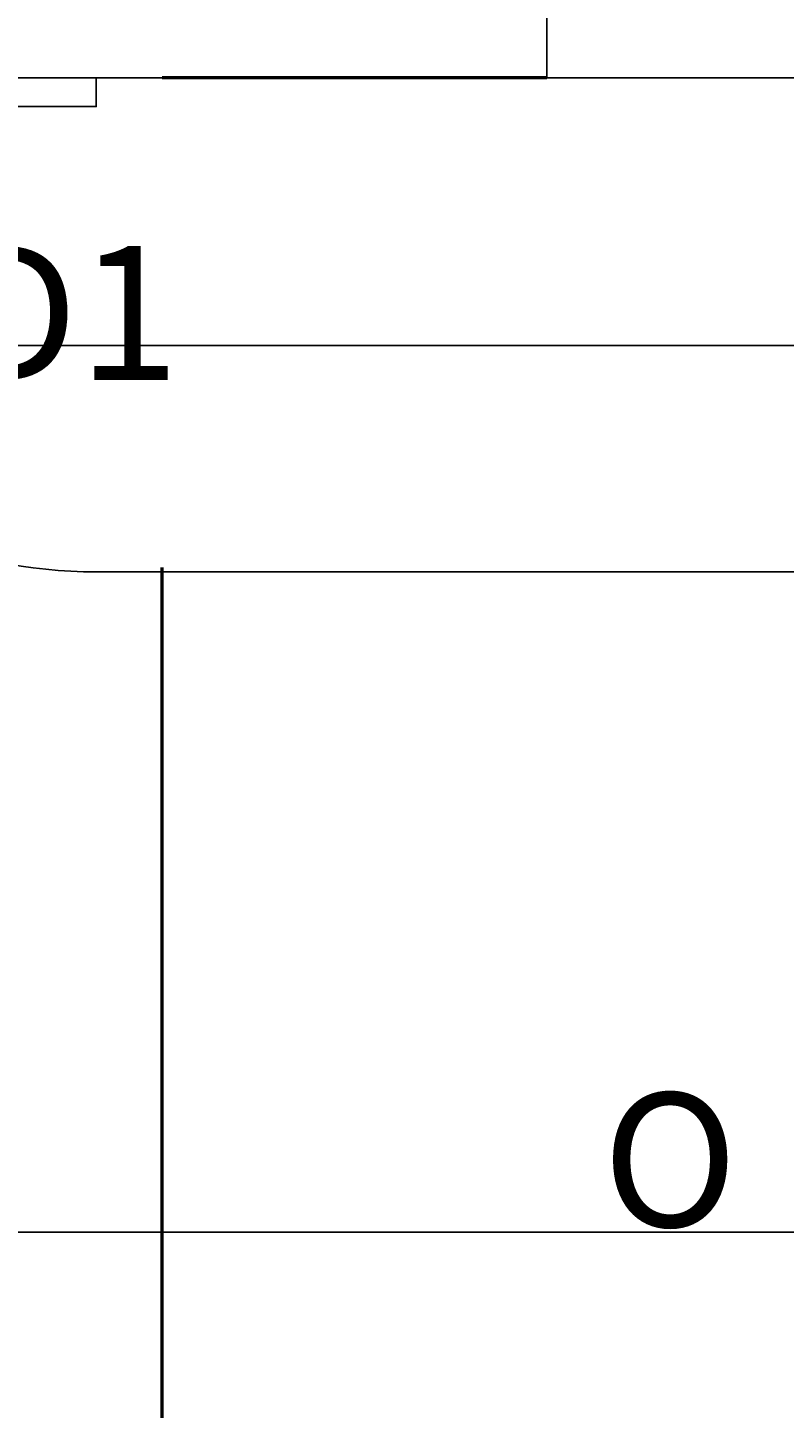
# Model space of a CAD drawing. Units: inches. Extents: x 37 to 824, y -700 to 234.
# Tile 48 of 77: x 219 to 264, y -4 to 78. Entities that reach past the tile are written whole.
import ezdxf

# ---------------------------------------------------------------- set-up
doc = ezdxf.new("R2010")
doc.units = ezdxf.units.IN
doc.header["$MEASUREMENT"] = 0
for name, color, linetype, lineweight in [('A-ANNO-DIMS', 2, 'Continuous', 18), ('A-ANNO-TEXT', 7, 'Continuous', 18), ('A-DOOR', 4, 'Continuous', 25), ('A-WALL', 2, 'Continuous', 50)]:
    doc.layers.add(name, color=color, linetype=linetype, lineweight=lineweight)
doc.styles.get("Standard").update_dxf_attribs({"font": 'arial.ttf'})
doc.dimstyles.get("Standard").update_dxf_attribs({"dimtxt": 0.18, "dimasz": 0.18, "dimexe": 0.18, "dimexo": 0.0625, "dimgap": 0.09, "dimtad": 0, "dimtih": 1, "dimtoh": 1, "dimdec": 1, "dimzin": 0, "dimdsep": 46, "dimlunit": 4, "dimtxsty": 'Standard', "dimcen": 0.09, "dimadec": 0, "dimazin": 0, "dimtfac": 1, "dimtdec": 1, "dimtofl": 0, "dimtmove": 0, "dimatfit": 3, "dimfxl": 1, "dimtolj": 1, "dimtzin": 0, "dimarcsym": 0})

# ---------------------------------------------------------------- blocks, each defined once
blk = doc.blocks.new('*U6')
for p, q in [((-750, 0), (-750, -100)), ((0, 0), (0, -100))]:
    blk.add_line(p, q)
blk.add_lwpolyline([(0, 0), (0, 750), (-43.75, 750), (-43.75, 0)], close=True)
blk.add_arc((0, 0), 750, 90, 180)
blk = doc.blocks.new('*U5')
for p, q in [((0, 0), (0, 6)), ((40, 0), (40, 6))]:
    blk.add_line(p, q)
blk.add_lwpolyline([(0, 0), (0, -40), (1.75, -40), (1.75, 0)], close=True)
blk.add_arc((0, 0), 40, 270, 0)
blk = doc.blocks.new('*D61')
at = {"layer": 'A-ANNO-DIMS', "color": 0, "lineweight": -2, "ltscale": 0.5, "transparency": 16777216}
for p, q in [((419.015, 75.09), (78.159, 75.09)), ((78.339, 74.91), (78.339, 67.271)), ((78.339, 59.27), (78.339, 66.91)), ((419.015, 59.09), (78.159, 59.09))]:
    blk.add_line(p, q, dxfattribs=at)
at = {"layer": 'A-ANNO-DIMS', "color": 0, "ltscale": 0.5, "transparency": 16777216}
for points in [[(78.309, 74.91), (78.369, 74.91), (78.339, 75.09)], [(78.309, 59.27), (78.369, 59.27), (78.339, 59.09)]]:
    blk.add_solid(points, dxfattribs=at)
at = {"layer": 'Defpoints', "color": 0, "ltscale": 0.5, "transparency": 16777216}
for p in [(419.077, 75.09), (78.339, 59.09), (419.077, 59.09)]:
    blk.add_point(p, dxfattribs=at)
at = {"layer": 'A-ANNO-DIMS', "color": 0, "ltscale": 0.5, "transparency": 16777216, "insert": (78.339, 67.09), "char_height": 0.18, "attachment_point": 5}
blk.add_mtext('\\A1;1\'-4"', dxfattribs=at)
blk = doc.blocks.new('*D62')
at = {"layer": 'A-ANNO-DIMS', "color": 0, "lineweight": -2, "ltscale": 0.5, "transparency": 16777216}
for p, q in [((419.015, 6.09), (78.159, 6.09)), ((78.339, 5.91), (78.339, -10.728)), ((78.339, -27.73), (78.339, -11.091)), ((419.015, -27.91), (78.159, -27.91))]:
    blk.add_line(p, q, dxfattribs=at)
at = {"layer": 'A-ANNO-DIMS', "color": 0, "ltscale": 0.5, "transparency": 16777216}
for points in [[(78.309, 5.91), (78.369, 5.91), (78.339, 6.09)], [(78.309, -27.73), (78.369, -27.73), (78.339, -27.91)]]:
    blk.add_solid(points, dxfattribs=at)
at = {"layer": 'Defpoints', "color": 0, "ltscale": 0.5, "transparency": 16777216}
for p in [(419.077, 6.09), (78.339, -27.91), (419.077, -27.91)]:
    blk.add_point(p, dxfattribs=at)
at = {"layer": 'A-ANNO-DIMS', "color": 0, "ltscale": 0.5, "transparency": 16777216, "insert": (78.339, -10.91), "char_height": 0.18, "attachment_point": 5}
blk.add_mtext('\\A1;2\'-10"', dxfattribs=at)
blk = doc.blocks.new('*D76')
at = {"layer": 'A-ANNO-DIMS', "color": 0, "lineweight": -2, "ltscale": 0.5, "transparency": 16777216}
for p, q in [((227.14, 75.09), (513.773, 75.09)), ((513.593, 74.91), (513.593, 60.51)), ((513.593, 45.743), (513.593, 60.144)), ((227.14, 45.563), (513.773, 45.563))]:
    blk.add_line(p, q, dxfattribs=at)
at = {"layer": 'A-ANNO-DIMS', "color": 0, "ltscale": 0.5, "transparency": 16777216}
for points in [[(513.563, 74.91), (513.623, 74.91), (513.593, 75.09)], [(513.563, 45.743), (513.623, 45.743), (513.593, 45.563)]]:
    blk.add_solid(points, dxfattribs=at)
at = {"layer": 'Defpoints', "color": 0, "ltscale": 0.5, "transparency": 16777216}
for p in [(227.077, 75.09), (227.077, 45.563), (513.593, 45.563)]:
    blk.add_point(p, dxfattribs=at)
at = {"layer": 'A-ANNO-DIMS', "color": 0, "ltscale": 0.5, "transparency": 16777216, "insert": (513.593, 60.327), "char_height": 0.18, "attachment_point": 5}
blk.add_mtext('\\A1;2\'-5 1/2"', dxfattribs=at)
blk = doc.blocks.new('*D77')
at = {"layer": 'A-ANNO-DIMS', "color": 0, "lineweight": -2, "ltscale": 0.5, "transparency": 16777216}
for p, q in [((227.077, 45.5), (227.077, -400.406)), ((290.077, 15.028), (290.077, -400.406)), ((227.257, -400.226), (258.248, -400.226)), ((289.897, -400.226), (258.906, -400.226))]:
    blk.add_line(p, q, dxfattribs=at)
at = {"layer": 'A-ANNO-DIMS', "color": 0, "ltscale": 0.5, "transparency": 16777216}
for points in [[(227.257, -400.196), (227.257, -400.256), (227.077, -400.226)], [(289.897, -400.196), (289.897, -400.256), (290.077, -400.226)]]:
    blk.add_solid(points, dxfattribs=at)
at = {"layer": 'Defpoints', "color": 0, "ltscale": 0.5, "transparency": 16777216}
for p in [(227.077, 45.563), (290.077, 15.09), (290.077, -400.226)]:
    blk.add_point(p, dxfattribs=at)
at = {"layer": 'A-ANNO-DIMS', "color": 0, "ltscale": 0.5, "transparency": 16777216, "insert": (258.577, -400.226), "char_height": 0.18, "attachment_point": 5}
blk.add_mtext('\\A1;5\'-3"', dxfattribs=at)
blk = doc.blocks.new('*D87')
at = {"layer": 'A-ANNO-DIMS', "color": 0, "lineweight": -2, "ltscale": 0.5, "transparency": 16777216}
for p, q in [((216.077, -356.847), (216.077, 234.17)), ((216.257, 233.99), (255.747, 233.99)), ((295.897, 233.99), (256.407, 233.99)), ((296.077, -356.847), (296.077, 234.17))]:
    blk.add_line(p, q, dxfattribs=at)
at = {"layer": 'A-ANNO-DIMS', "color": 0, "ltscale": 0.5, "transparency": 16777216}
for points in [[(216.257, 234.02), (216.257, 233.96), (216.077, 233.99)], [(295.897, 234.02), (295.897, 233.96), (296.077, 233.99)]]:
    blk.add_solid(points, dxfattribs=at)
at = {"layer": 'Defpoints', "color": 0, "ltscale": 0.5, "transparency": 16777216}
for p in [(296.077, 233.99), (216.077, -356.91), (296.077, -356.91)]:
    blk.add_point(p, dxfattribs=at)
at = {"layer": 'A-ANNO-DIMS', "color": 0, "ltscale": 0.5, "transparency": 16777216, "insert": (256.077, 233.99), "char_height": 0.18, "attachment_point": 5}
blk.add_mtext('\\A1;6\'-8"', dxfattribs=at)

msp = doc.modelspace()

# ---------------------------------------------------------------- linework, layer by layer
at = {"layer": 'A-WALL'}
for p, q in [((250.077, 75.09), (227.077, 75.09)), ((227.077, -11.91), (227.077, 45.826))]:
    msp.add_line(p, q, dxfattribs=at)

# ---------------------------------------------------------------- block references
at = {"layer": 'A-DOOR', "rotation": 180}
msp.add_blockref('*U5', (290.077, 81.09), dxfattribs=at)
at = {"layer": 'A-DOOR', "xscale": 0.0393700787401575, "yscale": 0.0393700787401575, "zscale": 0.0393700787401575, "rotation": 90}
msp.add_blockref('*U6', (223.14, 75.09), dxfattribs=at)

# ---------------------------------------------------------------- texts
at = {"layer": 'A-ANNO-TEXT'}
for s, p in [('D1', (214.553, 57.037)), ('O', (253.402, 6.417))]:
    msp.add_text(s, height=8, dxfattribs=at).set_placement(p)

# ---------------------------------------------------------------- dimensions: what is measured, and where the dimension line sits
at = {"layer": 'A-ANNO-DIMS', "ltscale": 0.5}
for base, p1, p2, picture, middle in [((296.077, 233.99), (216.077, -356.91), (296.077, -356.91), '*D87', (256.077, 233.99)), ((290.077, -400.226), (227.077, 45.563), (290.077, 15.09), '*D77', (258.577, -400.226))]:
    dim = msp.add_linear_dim(base=base, p1=p1, p2=p2, dimstyle='Standard', override={"dimdec": 1, "dimlfac": 1, "dimrnd": 0, "dimzin": 1, "dimdsep": 46, "dimlunit": 4, "dimfrac": 2}, dxfattribs=at)
    dim.commit()
    dim.dimension.update_dxf_attribs({"geometry": picture, "text_midpoint": middle})
for base, p1, p2, picture, middle in [((78.339, 59.09), (419.077, 75.09), (419.077, 59.09), '*D61', (78.339, 67.09)), ((513.593, 45.563), (227.077, 75.09), (227.077, 45.563), '*D76', (513.593, 60.327)), ((78.339, -27.91), (419.077, 6.09), (419.077, -27.91), '*D62', (78.339, -10.91))]:
    dim = msp.add_linear_dim(base=base, p1=p1, p2=p2, angle=90, dimstyle='Standard', override={"dimdec": 1, "dimlfac": 1, "dimrnd": 0, "dimzin": 1, "dimdsep": 46, "dimlunit": 4, "dimfrac": 2}, dxfattribs=at)
    dim.commit()
    dim.dimension.update_dxf_attribs({"geometry": picture, "text_midpoint": middle})

doc.saveas('drawing.dxf')
